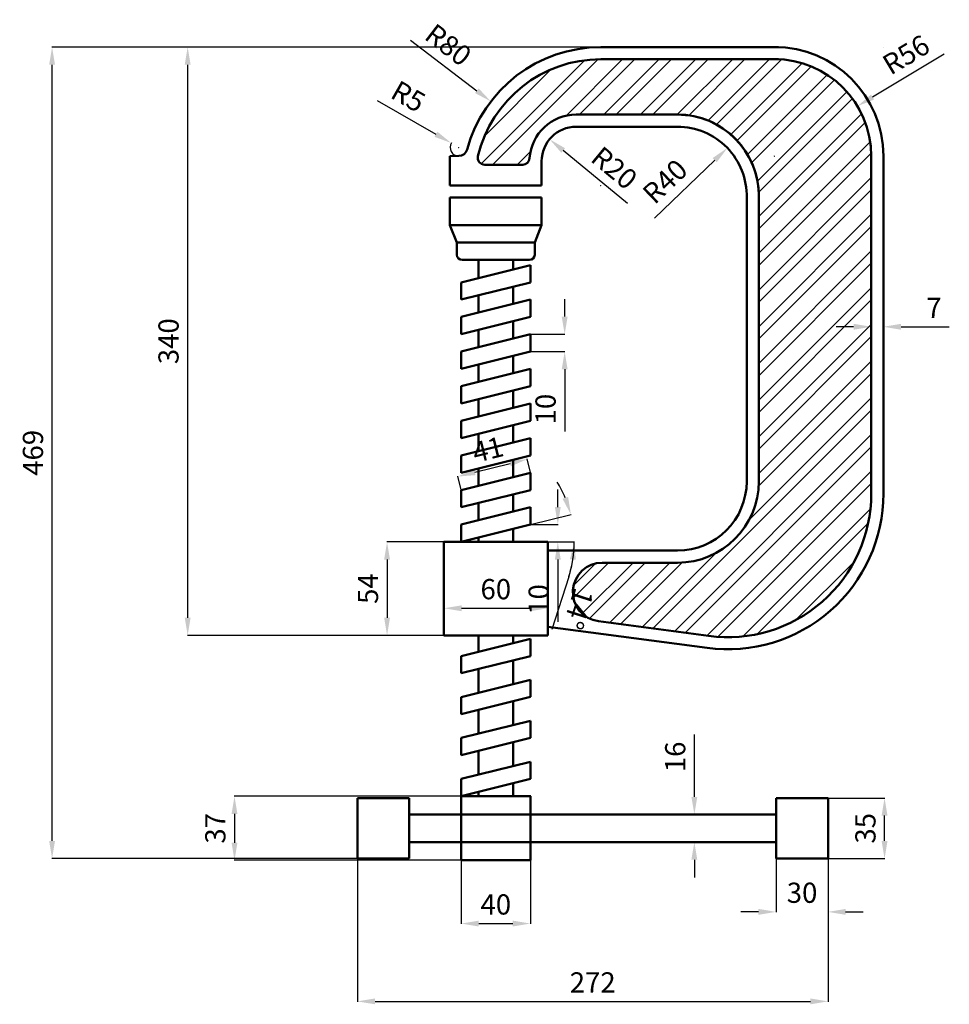
# Model space of a CAD drawing. Units: millimetres. Extents: x 725 to 1263, y 294 to 863.
import ezdxf

# ---------------------------------------------------------------- set-up
doc = ezdxf.new("R2010")
doc.units = ezdxf.units.MM
doc.header["$MEASUREMENT"] = 0
for name, color, linetype, lineweight in [('M-DIMS', 2, 'Continuous', 25), ('M-HATC', 8, 'Continuous', 18), ('M-OUTL', 7, 'Continuous', 50)]:
    doc.layers.add(name, color=color, linetype=linetype, lineweight=lineweight)
doc.styles.get("Standard").update_dxf_attribs({"font": 'arial.ttf'})
doc.dimstyles.get("Standard").update_dxf_attribs({"dimtxt": 11.68, "dimasz": 10.18, "dimexe": 0.18, "dimexo": 0.0625, "dimgap": 5.09, "dimtad": 1, "dimdec": 0, "dimzin": 0, "dimdsep": 46, "dimtxsty": 'Standard', "dimcen": 0.09, "dimclrd": 253, "dimclre": 253, "dimadec": 0, "dimazin": 0, "dimtfac": 1, "dimtdec": 0, "dimtofl": 0, "dimtmove": 0, "dimatfit": 3, "dimfxl": 1, "dimtolj": 1, "dimtzin": 0, "dimarcsym": 0})

# ---------------------------------------------------------------- blocks, each defined once
blk = doc.blocks.new('*U1')
for p, q in [((0.01, 20.05), (9.99, -20.06)), ((0.01, 20.05), (10.01, 20.05)), ((10.01, 20.05), (19.99, -20.07)), ((9.99, -20.06), (19.99, -20.07))]:
    blk.add_line(p, q)
blk = doc.blocks.new('*U2')
at = {"layer": 'M-OUTL', "color": 0, "linetype": 'ByBlock', "lineweight": -2, "transparency": 16777216, "rotation": 90.03320978073344}
for p in [(1000.56, 485.58), (1000.57, 461.89), (1000.59, 438.2), (1000.6, 414.51)]:
    blk.add_blockref('*U1', p, dxfattribs=at)
blk = doc.blocks.new('*D3')
at = {"layer": 'Defpoints', "color": 0, "lineweight": 25, "transparency": 16777216}
for p in [(920.55, 378.51), (1192.55, 378.51), (1192.55, 295.99)]:
    blk.add_point(p, dxfattribs=at)
at = {"layer": 'M-DIMS', "color": 0, "lineweight": -2, "transparency": 16777216}
for p, q in [((920.55, 378.45), (920.55, 295.81)), ((1192.55, 378.45), (1192.55, 295.81)), ((930.73, 295.99), (1182.37, 295.99))]:
    blk.add_line(p, q, dxfattribs=at)
at = {"layer": 'M-DIMS', "color": 0, "lineweight": 25, "transparency": 16777216}
for points in [[(930.73, 297.69), (930.73, 294.3), (920.55, 295.99)], [(1182.37, 297.69), (1182.37, 294.3), (1192.55, 295.99)]]:
    blk.add_solid(points, dxfattribs=at)
at = {"layer": 'M-DIMS', "color": 0, "transparency": 16777216, "insert": (1056.55, 306.95), "char_height": 11.68, "attachment_point": 5}
blk.add_mtext('\\A1;272', dxfattribs=at)
blk = doc.blocks.new('*D4')
at = {"layer": 'Defpoints', "color": 0, "lineweight": 25, "transparency": 16777216}
for p in [(980.55, 378.51), (1020.55, 377.51), (1020.55, 340.96)]:
    blk.add_point(p, dxfattribs=at)
at = {"layer": 'M-DIMS', "color": 0, "lineweight": -2, "transparency": 16777216}
for p, q in [((980.55, 378.45), (980.55, 340.78)), ((1020.55, 377.45), (1020.55, 340.78)), ((990.73, 340.96), (1010.37, 340.96))]:
    blk.add_line(p, q, dxfattribs=at)
at = {"layer": 'M-DIMS', "color": 0, "lineweight": 25, "transparency": 16777216}
for points in [[(990.73, 342.66), (990.73, 339.26), (980.55, 340.96)], [(1010.37, 342.66), (1010.37, 339.26), (1020.55, 340.96)]]:
    blk.add_solid(points, dxfattribs=at)
at = {"layer": 'M-DIMS', "color": 0, "transparency": 16777216, "insert": (1000.55, 352.01), "char_height": 11.68, "attachment_point": 5}
blk.add_mtext('\\A1;40', dxfattribs=at)
blk = doc.blocks.new('*D5')
at = {"layer": 'Defpoints', "color": 0, "lineweight": 25, "transparency": 16777216}
for p in [(1162.55, 378.51), (1192.55, 378.51), (1192.55, 347.71)]:
    blk.add_point(p, dxfattribs=at)
at = {"layer": 'M-DIMS', "color": 0, "lineweight": -2, "transparency": 16777216}
for p, q in [((1162.55, 378.45), (1162.55, 347.53)), ((1192.55, 378.45), (1192.55, 347.53)), ((1152.37, 347.71), (1142.19, 347.71)), ((1202.73, 347.71), (1212.91, 347.71))]:
    blk.add_line(p, q, dxfattribs=at)
at = {"layer": 'M-DIMS', "color": 0, "lineweight": 25, "transparency": 16777216}
for points in [[(1152.37, 349.41), (1152.37, 346.02), (1162.55, 347.71)], [(1202.73, 349.41), (1202.73, 346.02), (1192.55, 347.71)]]:
    blk.add_solid(points, dxfattribs=at)
at = {"layer": 'M-DIMS', "color": 0, "transparency": 16777216, "insert": (1177.55, 358.77), "char_height": 11.68, "attachment_point": 5}
blk.add_mtext('\\A1;30', dxfattribs=at)
blk = doc.blocks.new('*D6')
at = {"layer": 'Defpoints', "color": 0, "lineweight": 25, "transparency": 16777216}
for p in [(1192.55, 413.51), (1225.23, 413.51), (1192.55, 378.51)]:
    blk.add_point(p, dxfattribs=at)
at = {"layer": 'M-DIMS', "color": 0, "lineweight": -2, "transparency": 16777216}
for p, q in [((1192.61, 413.51), (1225.41, 413.51)), ((1225.23, 388.69), (1225.23, 403.33)), ((1192.61, 378.51), (1225.41, 378.51))]:
    blk.add_line(p, q, dxfattribs=at)
at = {"layer": 'M-DIMS', "color": 0, "lineweight": 25, "transparency": 16777216}
for points in [[(1223.53, 403.33), (1226.92, 403.33), (1225.23, 413.51)], [(1223.53, 388.69), (1226.92, 388.69), (1225.23, 378.51)]]:
    blk.add_solid(points, dxfattribs=at)
at = {"layer": 'M-DIMS', "color": 0, "transparency": 16777216, "insert": (1214.17, 396.01), "char_height": 11.68, "attachment_point": 5, "rotation": 90}
blk.add_mtext('\\A1;35', dxfattribs=at)
blk = doc.blocks.new('*D7')
at = {"layer": 'Defpoints', "color": 0, "lineweight": 25, "transparency": 16777216}
for p in [(1115.29, 404.01), (1162.55, 404.01), (1162.55, 388.01)]:
    blk.add_point(p, dxfattribs=at)
at = {"layer": 'M-DIMS', "color": 0, "lineweight": -2, "transparency": 16777216}
for p, q in [((1115.29, 414.19), (1115.29, 450.18)), ((1162.49, 404.01), (1115.11, 404.01)), ((1162.49, 388.01), (1115.11, 388.01)), ((1115.29, 377.83), (1115.29, 367.65))]:
    blk.add_line(p, q, dxfattribs=at)
at = {"layer": 'M-DIMS', "color": 0, "lineweight": 25, "transparency": 16777216}
for points in [[(1113.59, 414.19), (1116.99, 414.19), (1115.29, 404.01)], [(1113.59, 377.83), (1116.99, 377.83), (1115.29, 388.01)]]:
    blk.add_solid(points, dxfattribs=at)
at = {"layer": 'M-DIMS', "color": 0, "transparency": 16777216, "insert": (1104.24, 437.27), "char_height": 11.68, "attachment_point": 5, "rotation": 90}
blk.add_mtext('\\A1;16', dxfattribs=at)
blk = doc.blocks.new('*D8')
at = {"layer": 'Defpoints', "color": 0, "lineweight": 25, "transparency": 16777216}
for p in [(1020.79, 414.51), (849.52, 377.51), (1020.55, 377.51)]:
    blk.add_point(p, dxfattribs=at)
at = {"layer": 'M-DIMS', "color": 0, "lineweight": -2, "transparency": 16777216}
for p, q in [((1020.73, 414.51), (849.34, 414.51)), ((849.52, 404.33), (849.52, 387.69)), ((1020.49, 377.51), (849.34, 377.51))]:
    blk.add_line(p, q, dxfattribs=at)
at = {"layer": 'M-DIMS', "color": 0, "lineweight": 25, "transparency": 16777216}
for points in [[(847.82, 404.33), (851.22, 404.33), (849.52, 414.51)], [(847.82, 387.69), (851.22, 387.69), (849.52, 377.51)]]:
    blk.add_solid(points, dxfattribs=at)
at = {"layer": 'M-DIMS', "color": 0, "transparency": 16777216, "insert": (838.46, 396.01), "char_height": 11.68, "attachment_point": 5, "rotation": 90}
blk.add_mtext('\\A1;37', dxfattribs=at)
blk = doc.blocks.new('*D9')
at = {"layer": 'Defpoints', "color": 0, "lineweight": 25, "transparency": 16777216}
for p in [(744.1, 847.47), (920.55, 847.47), (920.55, 378.51)]:
    blk.add_point(p, dxfattribs=at)
at = {"layer": 'M-DIMS', "color": 0, "lineweight": -2, "transparency": 16777216}
for p, q in [((920.49, 847.47), (743.92, 847.47)), ((744.1, 388.69), (744.1, 837.29)), ((920.49, 378.51), (743.92, 378.51))]:
    blk.add_line(p, q, dxfattribs=at)
at = {"layer": 'M-DIMS', "color": 0, "lineweight": 25, "transparency": 16777216}
for points in [[(742.4, 837.29), (745.79, 837.29), (744.1, 847.47)], [(742.4, 388.69), (745.79, 388.69), (744.1, 378.51)]]:
    blk.add_solid(points, dxfattribs=at)
at = {"layer": 'M-DIMS', "color": 0, "transparency": 16777216, "insert": (733.04, 612.99), "char_height": 11.68, "attachment_point": 5, "rotation": 90}
blk.add_mtext('\\A1;469', dxfattribs=at)
blk = doc.blocks.new('*D10')
at = {"layer": 'Defpoints', "color": 0, "lineweight": 25, "transparency": 16777216}
for p in [(1112.61, 847.47), (822.46, 507.51), (1030.55, 507.51)]:
    blk.add_point(p, dxfattribs=at)
at = {"layer": 'M-DIMS', "color": 0, "lineweight": -2, "transparency": 16777216}
for p, q in [((1112.54, 847.47), (822.28, 847.47)), ((822.46, 837.29), (822.46, 517.69)), ((1030.49, 507.51), (822.28, 507.51))]:
    blk.add_line(p, q, dxfattribs=at)
at = {"layer": 'M-DIMS', "color": 0, "lineweight": 25, "transparency": 16777216}
for points in [[(820.76, 837.29), (824.15, 837.29), (822.46, 847.47)], [(820.76, 517.69), (824.15, 517.69), (822.46, 507.51)]]:
    blk.add_solid(points, dxfattribs=at)
at = {"layer": 'M-DIMS', "color": 0, "transparency": 16777216, "insert": (811.4, 677.49), "char_height": 11.68, "attachment_point": 5, "rotation": 90}
blk.add_mtext('\\A1;340', dxfattribs=at)
blk = doc.blocks.new('*D11')
at = {"layer": 'Defpoints', "color": 0, "lineweight": 25, "transparency": 16777216}
for p in [(970.55, 561.51), (937.7, 507.51), (970.55, 507.51)]:
    blk.add_point(p, dxfattribs=at)
at = {"layer": 'M-DIMS', "color": 0, "lineweight": -2, "transparency": 16777216}
for p, q in [((970.49, 561.51), (937.52, 561.51)), ((937.7, 551.33), (937.7, 517.69)), ((970.49, 507.51), (937.52, 507.51))]:
    blk.add_line(p, q, dxfattribs=at)
at = {"layer": 'M-DIMS', "color": 0, "lineweight": 25, "transparency": 16777216}
for points in [[(936, 551.33), (939.4, 551.33), (937.7, 561.51)], [(936, 517.69), (939.4, 517.69), (937.7, 507.51)]]:
    blk.add_solid(points, dxfattribs=at)
at = {"layer": 'M-DIMS', "color": 0, "transparency": 16777216, "insert": (926.67, 534.51), "char_height": 11.68, "attachment_point": 5, "rotation": 90}
blk.add_mtext('\\A1;54', dxfattribs=at)
blk = doc.blocks.new('*D12')
at = {"layer": 'Defpoints', "color": 0, "lineweight": 25, "transparency": 16777216}
for p in [(970.55, 531.05), (1030.55, 534.51), (1030.55, 523.16)]:
    blk.add_point(p, dxfattribs=at)
at = {"layer": 'M-DIMS', "color": 0, "lineweight": -2, "transparency": 16777216}
for p, q in [((970.55, 530.99), (970.55, 522.98)), ((1030.55, 534.45), (1030.55, 522.98)), ((980.73, 523.16), (1020.37, 523.16))]:
    blk.add_line(p, q, dxfattribs=at)
at = {"layer": 'M-DIMS', "color": 0, "lineweight": 25, "transparency": 16777216}
for points in [[(980.73, 524.85), (980.73, 521.46), (970.55, 523.16)], [(1020.37, 524.85), (1020.37, 521.46), (1030.55, 523.16)]]:
    blk.add_solid(points, dxfattribs=at)
at = {"layer": 'M-DIMS', "color": 0, "transparency": 16777216, "insert": (1000.55, 534.21), "char_height": 11.68, "attachment_point": 5}
blk.add_mtext('\\A1;60', dxfattribs=at)
blk = doc.blocks.new('*D13')
at = {"layer": 'Defpoints', "color": 0, "lineweight": 25, "transparency": 16777216}
for p in [(1020.6, 571.51), (1045.03, 572.12), (980.49, 561.51), (980.49, 561.51), (1020.6, 561.51)]:
    blk.add_point(p, dxfattribs=at)
at = {"layer": 'M-DIMS', "color": 0, "lineweight": -2, "transparency": 16777216}
for p, q in [((1020.66, 571.53), (1044.13, 577.38)), ((1020.66, 561.51), (1046.08, 561.51)), ((1042.73, 541.4), (1032.89, 510.96))]:
    blk.add_line(p, q, dxfattribs=at)
for start, end in [(22.927, 31.8541), (342.0912, 360), (342.1459, 351.073)]:
    blk.add_arc((980.49, 561.51), 65.4, start, end, dxfattribs=at)
at = {"layer": 'M-DIMS', "color": 0, "lineweight": 25, "transparency": 16777216}
for points in [[(1042.34, 587.53), (1039.12, 586.45), (1043.96, 577.33)], [(1043.41, 551.5), (1046.8, 551.23), (1045.9, 561.51)]]:
    blk.add_solid(points, dxfattribs=at)
at = {"layer": 'M-DIMS', "color": 0, "transparency": 16777216, "insert": (1048.23, 522.81), "char_height": 11.68, "attachment_point": 5, "rotation": 252.0912}
blk.add_mtext('\\A1;14°', dxfattribs=at)
blk = doc.blocks.new('*D14')
at = {"layer": 'Defpoints', "color": 0, "lineweight": 25, "transparency": 16777216}
for p in [(1020.6, 571.51), (1020.74, 561.51), (1036.38, 561.51)]:
    blk.add_point(p, dxfattribs=at)
at = {"layer": 'M-DIMS', "color": 0, "lineweight": -2, "transparency": 16777216}
for p, q in [((1036.38, 581.69), (1036.38, 591.87)), ((1020.66, 571.51), (1036.56, 571.51)), ((1020.8, 561.51), (1036.56, 561.51)), ((1036.38, 551.33), (1036.38, 515.38))]:
    blk.add_line(p, q, dxfattribs=at)
at = {"layer": 'M-DIMS', "color": 0, "lineweight": 25, "transparency": 16777216}
for points in [[(1034.69, 581.69), (1038.08, 581.69), (1036.38, 571.51)], [(1034.69, 551.33), (1038.08, 551.33), (1036.38, 561.51)]]:
    blk.add_solid(points, dxfattribs=at)
at = {"layer": 'M-DIMS', "color": 0, "transparency": 16777216, "insert": (1025.33, 528.27), "char_height": 11.68, "attachment_point": 5, "rotation": 90}
blk.add_mtext('\\A1;10', dxfattribs=at)
blk = doc.blocks.new('*D15')
at = {"layer": 'Defpoints', "color": 0, "lineweight": 25, "transparency": 16777216}
for p in [(1018.66, 609.29), (1020.6, 601.51), (980.49, 591.51)]:
    blk.add_point(p, dxfattribs=at)
at = {"layer": 'M-DIMS', "color": 0, "lineweight": -2, "transparency": 16777216}
for p, q in [((1020.59, 601.57), (1018.62, 609.47)), ((988.43, 601.75), (1008.78, 606.83)), ((980.48, 591.57), (978.51, 599.47))]:
    blk.add_line(p, q, dxfattribs=at)
at = {"layer": 'M-DIMS', "color": 0, "lineweight": 25, "transparency": 16777216}
for points in [[(1008.37, 608.48), (1009.2, 605.18), (1018.66, 609.29)], [(988.02, 603.4), (988.84, 600.11), (978.55, 599.29)]]:
    blk.add_solid(points, dxfattribs=at)
at = {"layer": 'M-DIMS', "color": 0, "transparency": 16777216, "insert": (995.96, 614.92), "char_height": 11.68, "attachment_point": 5, "rotation": 14}
blk.add_mtext('\\A1;41', dxfattribs=at)
blk = doc.blocks.new('*D16')
at = {"layer": 'Defpoints', "color": 0, "lineweight": 25, "transparency": 16777216}
for p in [(1020.6, 681.51), (1020.6, 671.51), (1040.35, 671.51)]:
    blk.add_point(p, dxfattribs=at)
at = {"layer": 'M-DIMS', "color": 0, "lineweight": -2, "transparency": 16777216}
for p, q in [((1040.35, 691.69), (1040.35, 701.87)), ((1020.66, 681.51), (1040.53, 681.51)), ((1020.66, 671.51), (1040.53, 671.51)), ((1040.35, 661.33), (1040.35, 625.38))]:
    blk.add_line(p, q, dxfattribs=at)
at = {"layer": 'M-DIMS', "color": 0, "lineweight": 25, "transparency": 16777216}
for points in [[(1038.65, 691.69), (1042.05, 691.69), (1040.35, 681.51)], [(1038.65, 661.33), (1042.05, 661.33), (1040.35, 671.51)]]:
    blk.add_solid(points, dxfattribs=at)
at = {"layer": 'M-DIMS', "color": 0, "transparency": 16777216, "insert": (1029.3, 638.27), "char_height": 11.68, "attachment_point": 5, "rotation": 90}
blk.add_mtext('\\A1;10', dxfattribs=at)
blk = doc.blocks.new('*D17')
at = {"layer": 'Defpoints', "color": 0, "lineweight": 25, "transparency": 16777216}
for p in [(1217.55, 686.96), (1224.55, 686.96), (1224.55, 685.85)]:
    blk.add_point(p, dxfattribs=at)
at = {"layer": 'M-DIMS', "color": 0, "lineweight": -2, "transparency": 16777216}
for p, q in [((1207.37, 685.85), (1197.19, 685.85)), ((1217.55, 686.9), (1217.55, 685.67)), ((1224.55, 686.9), (1224.55, 685.67)), ((1234.73, 685.85), (1262.65, 685.85))]:
    blk.add_line(p, q, dxfattribs=at)
at = {"layer": 'M-DIMS', "color": 0, "lineweight": 25, "transparency": 16777216}
for points in [[(1207.37, 687.54), (1207.37, 684.15), (1217.55, 685.85)], [(1234.73, 687.54), (1234.73, 684.15), (1224.55, 685.85)]]:
    blk.add_solid(points, dxfattribs=at)
at = {"layer": 'M-DIMS', "color": 0, "transparency": 16777216, "insert": (1253.78, 696.78), "char_height": 11.68, "attachment_point": 5}
blk.add_mtext('\\A1;7', dxfattribs=at)
blk = doc.blocks.new('*D18')
at = {"layer": 'Defpoints', "color": 0, "lineweight": 25, "transparency": 16777216}
for p in [(1209.56, 813.34), (1161.55, 784.51)]:
    blk.add_point(p, dxfattribs=at)
at = {"layer": 'M-DIMS', "color": 0, "lineweight": -2, "transparency": 16777216}
for p, q in [((1259.66, 843.42), (1218.29, 818.58)), ((1161.46, 784.51), (1161.64, 784.51)), ((1161.55, 784.42), (1161.55, 784.6))]:
    blk.add_line(p, q, dxfattribs=at)
at = {"layer": 'M-DIMS', "color": 0, "lineweight": 25, "transparency": 16777216}
blk.add_solid([(1217.41, 820.03), (1219.16, 817.12), (1209.56, 813.34)], dxfattribs=at)
at = {"layer": 'M-DIMS', "color": 0, "transparency": 16777216, "insert": (1237.65, 843.1), "char_height": 11.68, "attachment_point": 5, "rotation": 30.9806}
blk.add_mtext('\\A1;R56', dxfattribs=at)
blk = doc.blocks.new('*D19')
at = {"layer": 'Defpoints', "color": 0, "lineweight": 25, "transparency": 16777216}
for p in [(997.68, 816.06), (1061.22, 767.47)]:
    blk.add_point(p, dxfattribs=at)
at = {"layer": 'M-DIMS', "color": 0, "lineweight": -2, "transparency": 16777216}
for p, q in [((951.28, 851.55), (989.59, 822.25)), ((1061.13, 767.47), (1061.31, 767.47)), ((1061.22, 767.38), (1061.22, 767.56))]:
    blk.add_line(p, q, dxfattribs=at)
at = {"layer": 'M-DIMS', "color": 0, "lineweight": 25, "transparency": 16777216}
blk.add_solid([(990.62, 823.6), (988.56, 820.9), (997.68, 816.06)], dxfattribs=at)
at = {"layer": 'M-DIMS', "color": 0, "transparency": 16777216, "insert": (973.11, 848.77), "char_height": 11.68, "attachment_point": 5, "rotation": 322.5916}
blk.add_mtext('\\A1;R80', dxfattribs=at)
blk = doc.blocks.new('*D20')
at = {"layer": 'Defpoints', "color": 0, "lineweight": 25, "transparency": 16777216}
for p in [(974.8, 792.03), (979.14, 789.54)]:
    blk.add_point(p, dxfattribs=at)
at = {"layer": 'M-DIMS', "color": 0, "lineweight": -2, "transparency": 16777216}
for p, q in [((931.89, 816.62), (965.97, 797.09)), ((979.05, 789.54), (979.23, 789.54)), ((979.14, 789.45), (979.14, 789.63))]:
    blk.add_line(p, q, dxfattribs=at)
blk.add_arc((979.14, 789.54), 5, 148.1192, 269.2838, dxfattribs=at)
at = {"layer": 'M-DIMS', "color": 0, "lineweight": 25, "transparency": 16777216}
blk.add_solid([(966.81, 798.56), (965.13, 795.62), (974.8, 792.03)], dxfattribs=at)
at = {"layer": 'M-DIMS', "color": 0, "transparency": 16777216, "insert": (950, 818.96), "char_height": 11.68, "attachment_point": 5, "rotation": 330.1819}
blk.add_mtext('\\A1;R5', dxfattribs=at)
blk = doc.blocks.new('*D21')
at = {"layer": 'Defpoints', "color": 0, "lineweight": 25, "transparency": 16777216}
for p in [(1031.63, 794.21), (1047.05, 781.47)]:
    blk.add_point(p, dxfattribs=at)
at = {"layer": 'M-DIMS', "color": 0, "lineweight": -2, "transparency": 16777216}
blk.add_line((1076.65, 756.99), (1039.48, 787.72), dxfattribs=at)
at = {"layer": 'M-DIMS', "color": 0, "lineweight": 25, "transparency": 16777216}
blk.add_solid([(1040.56, 789.03), (1038.4, 786.41), (1031.63, 794.21)], dxfattribs=at)
at = {"layer": 'M-DIMS', "color": 0, "transparency": 16777216, "insert": (1069.03, 777.64), "char_height": 11.68, "attachment_point": 5, "rotation": 320.4249}
blk.add_mtext('\\A1;R20', dxfattribs=at)
blk = doc.blocks.new('*D22')
at = {"layer": 'Defpoints', "color": 0, "lineweight": 25, "transparency": 16777216}
for p in [(1134.39, 789.18), (1105.54, 761.44)]:
    blk.add_point(p, dxfattribs=at)
at = {"layer": 'M-DIMS', "color": 0, "lineweight": -2, "transparency": 16777216}
blk.add_line((1092.28, 748.7), (1127.05, 782.13), dxfattribs=at)
at = {"layer": 'M-DIMS', "color": 0, "lineweight": 25, "transparency": 16777216}
blk.add_solid([(1125.87, 783.35), (1128.23, 780.9), (1134.39, 789.18)], dxfattribs=at)
at = {"layer": 'M-DIMS', "color": 0, "transparency": 16777216, "insert": (1098.34, 769.85), "char_height": 11.68, "attachment_point": 5, "rotation": 43.8747}
blk.add_mtext('\\A1;R40', dxfattribs=at)

msp = doc.modelspace()

# ---------------------------------------------------------------- hatches: boundary and pattern name
at = {"layer": 'M-HATC'}
h = msp.add_hatch(dxfattribs=at)
h.set_pattern_fill('ANSI32', color=256, scale=40)
h.paths.add_polyline_path([(1163.85, 840.47), (1061.22, 840.47, 0.347022), (990.23, 784.44, 0.484757), (994.12, 779.51), (1016.12, 779.51, 0.394986), (1020.11, 783.25, -0.394986), (1047.05, 808.47), (1105.53, 808.47, -0.420901), (1152.55, 760.38), (1152.55, 596.51, -0.414214), (1105.55, 549.51), (1062.08, 549.51, 0.935703), (1059.83, 515.66), (1123.56, 507.15, 0.453672), (1217.55, 589.42), (1217.55, 784.51, 0.402225)])

# ---------------------------------------------------------------- linework, layer by layer
at = {"layer": 'M-OUTL'}
for p, q in [((1061.22, 847.47), (1163.99, 847.47)), ((1224.55, 847.51), (1224.55, 847.47)), ((1224.55, 847.47), (1224.55, 847.51)), ((1061.22, 840.47), (1163.99, 840.47)), ((1047.05, 808.47), (1105.55, 808.47)), ((1047.05, 801.47), (1105.55, 801.47)), ((974.05, 784.51), (979.19, 784.54)), ((974.05, 767.51), (974.05, 784.51)), ((1027.05, 767.51), (1027.05, 781.47)), ((1217.55, 784.51), (1217.55, 589.42)), ((1224.55, 666.6), (1224.55, 784.51)), ((1224.55, 784.51), (1224.55, 589.42)), ((974.05, 767.51), (974.05, 779.51)), ((994.12, 779.51), (1016.12, 779.51)), ((974.05, 767.51), (1027.05, 767.51)), ((1027.05, 760.51), (974.05, 760.51)), ((974.05, 760.51), (974.05, 744.51)), ((1027.05, 744.51), (1027.05, 760.51)), ((1145.55, 596.51), (1145.55, 760.47)), ((1152.55, 596.51), (1152.55, 760.47)), ((978.05, 734.51), (974.05, 744.51)), ((974.05, 744.51), (1027.05, 744.51)), ((1023.05, 734.51), (1027.05, 744.51)), ((978.05, 734.51), (978.05, 727.51)), ((978.05, 734.51), (1023.05, 734.51)), ((1023.05, 727.51), (1023.05, 734.51)), ((981.05, 724.51), (1020.05, 724.51)), ((990.55, 724.51), (990.55, 714.02)), ((1010.55, 719.01), (1010.55, 724.51)), ((980.49, 711.51), (1020.6, 721.51)), ((1020.6, 711.51), (1020.6, 721.51)), ((980.49, 701.51), (1020.6, 711.51)), ((980.49, 701.51), (980.49, 711.51)), ((1010.55, 699.01), (1010.55, 709.01)), ((980.49, 691.51), (1020.6, 701.51)), ((990.55, 704.02), (990.55, 694.02)), ((1020.6, 691.51), (1020.6, 701.51)), ((980.49, 681.51), (1020.6, 691.51)), ((980.49, 681.51), (980.49, 691.51)), ((1010.55, 679.01), (1010.55, 689.01)), ((990.55, 684.02), (990.55, 674.02)), ((980.49, 671.51), (1020.6, 681.51)), ((1020.6, 671.51), (1020.6, 681.51)), ((980.49, 661.51), (1020.6, 671.51)), ((980.49, 661.51), (980.49, 671.51)), ((1010.55, 659.01), (1010.55, 669.01)), ((980.49, 651.51), (1020.6, 661.51)), ((990.55, 664.02), (990.55, 654.02)), ((1020.6, 651.51), (1020.6, 661.51)), ((980.49, 641.51), (1020.6, 651.51)), ((980.49, 641.51), (980.49, 651.51)), ((1010.55, 639.01), (1010.55, 649.01)), ((990.55, 644.02), (990.55, 634.02)), ((980.49, 631.51), (1020.6, 641.51)), ((1020.6, 631.51), (1020.6, 641.51)), ((980.49, 621.51), (1020.6, 631.51)), ((980.49, 621.51), (980.49, 631.51)), ((1010.55, 619.01), (1010.55, 629.01)), ((980.49, 611.51), (1020.6, 621.51)), ((990.55, 624.02), (990.55, 614.02)), ((1020.6, 611.51), (1020.6, 621.51)), ((980.49, 601.51), (1020.6, 611.51)), ((980.49, 601.51), (980.49, 611.51)), ((1010.55, 599.01), (1010.55, 609.01)), ((990.55, 604.02), (990.55, 594.02)), ((980.49, 591.51), (1020.6, 601.51)), ((1020.6, 591.51), (1020.6, 601.51)), ((980.49, 581.51), (1020.6, 591.51)), ((980.49, 581.51), (980.49, 591.51)), ((1010.55, 579.01), (1010.55, 589.01)), ((980.49, 571.51), (1020.6, 581.51)), ((990.55, 584.02), (990.55, 574.02)), ((1020.6, 571.51), (1020.6, 581.51)), ((980.49, 561.51), (1020.6, 571.51)), ((980.49, 561.51), (980.49, 571.51)), ((990.55, 564.02), (990.55, 561.51)), ((1010.55, 561.51), (1010.55, 569.01)), ((970.55, 507.51), (970.55, 561.51)), ((970.55, 561.51), (1030.55, 561.51)), ((980.36, 561.51), (1020.74, 561.51)), ((1020.6, 561.51), (980.49, 561.51)), ((1030.55, 561.51), (1030.55, 507.51)), ((1030.55, 534.51), (1030.55, 556.51)), ((1030.55, 556.51), (1105.55, 556.51)), ((1062.08, 549.51), (1105.55, 549.51)), ((1030.55, 512.51), (1122.63, 500.21)), ((1059.83, 515.66), (1123.56, 507.15)), ((1000.55, 507.51), (970.55, 507.51)), ((1030.55, 507.51), (970.55, 507.51)), ((1000.55, 507.51), (990.55, 507.51)), ((1010.55, 507.51), (990.55, 507.51)), ((990.55, 507.51), (990.55, 498.08)), ((1010.55, 503.07), (1010.55, 507.51)), ((990.55, 498.08), (990.55, 498.08)), ((1010.55, 479.38), (1010.55, 493.07)), ((990.55, 488.08), (990.55, 474.39)), ((1010.55, 455.68), (1010.55, 469.38)), ((990.55, 464.39), (990.55, 450.7)), ((1010.55, 431.99), (1010.55, 445.68)), ((990.55, 440.7), (990.55, 427.01)), ((1010.55, 414.51), (1010.55, 421.99)), ((990.55, 417.01), (990.55, 414.51)), ((950.55, 413.51), (920.55, 413.51)), ((920.55, 413.51), (920.55, 378.51)), ((950.55, 378.51), (950.55, 413.51)), ((950.55, 413.51), (950.55, 378.51)), ((980.41, 414.51), (1020.79, 414.51)), ((980.55, 396.01), (980.55, 414.51)), ((980.55, 414.51), (1020.55, 414.51)), ((980.55, 377.51), (980.55, 414.51)), ((1020.66, 414.51), (980.55, 414.51)), ((980.55, 378.51), (980.55, 413.51)), ((990.55, 414.51), (1010.55, 414.51)), ((1020.55, 414.51), (1020.55, 377.51)), ((1162.55, 378.51), (1162.55, 413.51)), ((1162.55, 413.51), (1192.55, 413.51)), ((1192.55, 413.51), (1192.55, 378.51)), ((920.55, 404.01), (920.55, 388.01)), ((1162.55, 404.01), (950.55, 404.01)), ((1192.55, 396.01), (1192.55, 404.01)), ((950.55, 388.01), (1162.55, 388.01)), ((920.55, 378.51), (950.55, 378.51)), ((1020.55, 377.51), (980.55, 377.51)), ((1192.55, 378.51), (1162.55, 378.51))]:
    msp.add_line(p, q, dxfattribs=at)
for centre, radius, start, end in [((1061.22, 767.47), 80, 90, 164.9463), ((1161.55, 784.51), 63, 0, 90), ((1061.22, 767.47), 73, 90, 166.5516), ((1161.55, 784.51), 56, 0, 90), ((1047.05, 781.47), 27, 90, 176.2133), ((1105.55, 761.47), 47, 0, 90), ((1105.54, 761.44), 47.02, 358.5975, 89.9879), ((1047.05, 781.47), 20, 90, 180), ((1105.54, 761.44), 40.02, 358.5975, 89.9879), ((979.14, 789.54), 5, 270, 344.9463), ((994.12, 783.51), 4, 166.5516, 270), ((1016.12, 783.51), 4, 270, 356.2133), ((981.05, 727.51), 3, 180, 270), ((1020.05, 727.51), 3, 270, 0), ((1105.55, 596.51), 40, 270, 0), ((1105.55, 596.51), 47, 270, 0), ((1134.55, 589.42), 90, 262.3902, 0), ((1134.55, 589.42), 83, 262.3902, 0), ((1062.08, 532.51), 17, 90, 262.3902)]:
    msp.add_arc(centre, radius, start, end, dxfattribs=at)

# ---------------------------------------------------------------- block references
msp.add_blockref('*U2', (0, 0), dxfattribs=at)

# ---------------------------------------------------------------- dimensions: what is measured, and where the dimension line sits
at = {"layer": 'M-DIMS'}
for center, mpoint, picture, middle in [((1061.22, 767.47), (997.68, 816.06), '*D19', (973.11, 848.77)), ((1161.55, 784.51), (1209.56, 813.34), '*D18', (1237.65, 843.1)), ((979.14, 789.54), (974.8, 792.03), '*D20', (950, 818.96))]:
    dim = msp.add_radius_dim(center=center, mpoint=mpoint, dimstyle='Standard', override={"dimclrd": 0, "dimclre": 0, "dimclrt": 0}, dxfattribs=at)
    dim.commit()
    dim.dimension.update_dxf_attribs({"geometry": picture, "text_midpoint": middle})
for base, p1, p2, picture, middle in [((744.1, 847.47), (920.55, 378.51), (920.55, 847.47), '*D9', (733.04, 612.99)), ((822.46, 507.51), (1112.61, 847.47), (1030.55, 507.51), '*D10', (811.4, 677.49)), ((1040.35, 671.51), (1020.6, 681.51), (1020.6, 671.51), '*D16', (1029.3, 638.27)), ((1036.38, 561.51), (1020.6, 571.51), (1020.74, 561.51), '*D14', (1025.33, 528.27)), ((937.7, 507.51), (970.55, 561.51), (970.55, 507.51), '*D11', (926.67, 534.51)), ((1115.29, 404.01), (1162.55, 388.01), (1162.55, 404.01), '*D7', (1104.24, 437.27)), ((849.52, 377.51), (1020.79, 414.51), (1020.55, 377.51), '*D8', (838.46, 396.01)), ((1225.23, 413.51), (1192.55, 378.51), (1192.55, 413.51), '*D6', (1214.17, 396.01))]:
    dim = msp.add_linear_dim(base=base, p1=p1, p2=p2, angle=90, dimstyle='Standard', override={"dimclrd": 0, "dimclre": 0, "dimclrt": 0}, dxfattribs=at)
    dim.commit()
    dim.dimension.update_dxf_attribs({"geometry": picture, "text_midpoint": middle})
for center, mpoint, picture, middle in [((1047.05, 781.47), (1031.63, 794.21), '*D21', (1061.99, 769.12)), ((1105.54, 761.44), (1134.39, 789.18), '*D22', (1106, 761.89))]:
    dim = msp.add_radius_dim(center=center, mpoint=mpoint, dimstyle='Standard', override={"dimclrd": 0, "dimclre": 0, "dimclrt": 0}, dxfattribs=at)
    dim.commit()
    dim.dimension.update_dxf_attribs({"geometry": picture, "text_midpoint": middle, "dimtype": 164})
for base, p1, p2, picture, middle in [((1224.55, 685.85), (1217.55, 686.96), (1224.55, 686.96), '*D17', (1253.78, 696.78)), ((1030.55, 523.16), (970.55, 531.05), (1030.55, 534.51), '*D12', (1000.55, 534.21)), ((1192.55, 295.99), (920.55, 378.51), (1192.55, 378.51), '*D3', (1056.55, 306.95)), ((1020.55, 340.96), (980.55, 378.51), (1020.55, 377.51), '*D4', (1000.55, 352.01)), ((1192.55, 347.71), (1162.55, 378.51), (1192.55, 378.51), '*D5', (1177.55, 358.77))]:
    dim = msp.add_linear_dim(base=base, p1=p1, p2=p2, dimstyle='Standard', override={"dimclrd": 0, "dimclre": 0, "dimclrt": 0}, dxfattribs=at)
    dim.commit()
    dim.dimension.update_dxf_attribs({"geometry": picture, "text_midpoint": middle})
dim = msp.add_aligned_dim(p1=(980.49, 591.51), p2=(1020.6, 601.51), distance=8.02, dimstyle='Standard', override={"dimclrd": 0, "dimclre": 0, "dimclrt": 0}, dxfattribs=at)
dim.commit()
dim.dimension.update_dxf_attribs({"geometry": '*D15', "text_midpoint": (995.96, 614.92)})
dim = msp.add_angular_dim_2l(base=(1045.03, 572.12), line1=((1020.6, 561.51), (980.49, 561.51)), line2=((980.49, 561.51), (1020.6, 571.51)), dimstyle='Standard', override={"dimclrd": 0, "dimclre": 0, "dimclrt": 0}, dxfattribs=at)
dim.commit()
dim.dimension.update_dxf_attribs({"geometry": '*D13', "text_midpoint": (1048.23, 522.81)})

doc.saveas('drawing.dxf')
